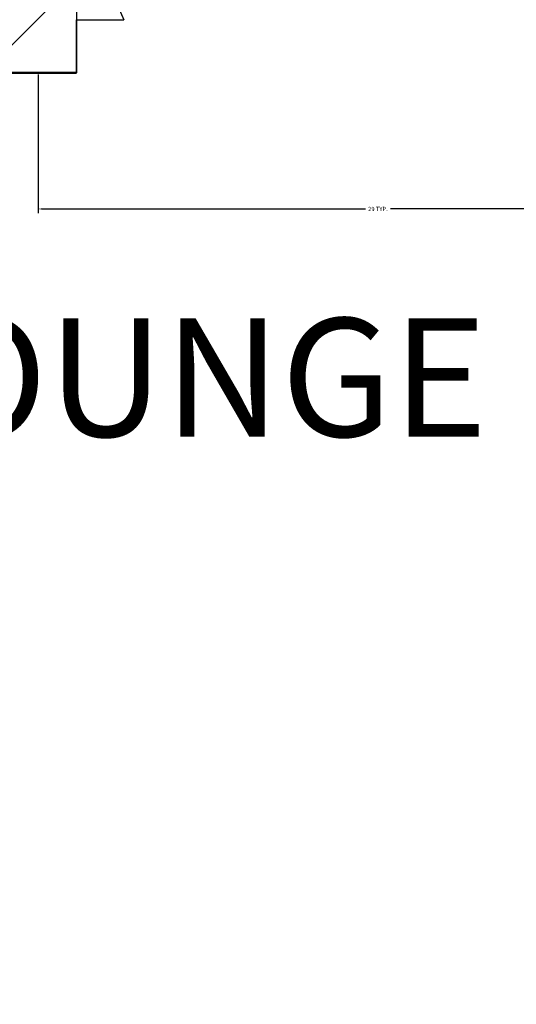
# Model space of a CAD drawing. Units: inches. Extents: x 963 to 2075, y 289 to 2657.
# Tile 64 of 98: x 1224 to 1245, y 2284 to 2325. Entities that reach past the tile are written whole.
import ezdxf

# ---------------------------------------------------------------- set-up
doc = ezdxf.new("R2010")
doc.units = ezdxf.units.IN
for name, color, linetype, lineweight in [('A-ANNO-DIMS', 2, 'Continuous', 18), ('A-AREA-IDEN', 7, 'Continuous', 18), ('A-DOOR', 4, 'Continuous', 25), ('A-WALL', 7, 'Continuous', 50), ('A-WALL-PATT', 8, 'Continuous', 13)]:
    doc.layers.add(name, color=color, linetype=linetype, lineweight=lineweight)
doc.styles.get("Standard").update_dxf_attribs({"font": 'arial.ttf'})
doc.dimstyles.get("Standard").update_dxf_attribs({"dimtxt": 0.18, "dimasz": 0.18, "dimexe": 0.18, "dimexo": 0.0625, "dimgap": 0.09, "dimtad": 0, "dimtih": 1, "dimtoh": 1, "dimdec": 4, "dimzin": 0, "dimdsep": 46, "dimtxsty": 'Standard', "dimcen": 0.09, "dimadec": 0, "dimazin": 0, "dimtfac": 1, "dimtdec": 4, "dimtofl": 0, "dimtmove": 0, "dimatfit": 3, "dimfxl": 1, "dimtolj": 1, "dimtzin": 0, "dimarcsym": 0})

# ---------------------------------------------------------------- blocks, each defined once
blk = doc.blocks.new('DOOR-1')
for p, q in [((25.385, 2.25), (25.385, 38.25)), ((0.325, 4.5), (0.325, 0)), ((27.385, 4.5), (27.385, 0)), ((0.325, 0), (0.325, 2.25)), ((0.325, 2.25), (2.325, 2.25)), ((27.385, 2.25), (25.385, 2.25)), ((27.385, 0), (27.385, 2.25))]:
    blk.add_line(p, q)
blk.add_arc((25.385, 12.864), 25.386, 90, 204.7158)
blk = doc.blocks.new('*D31')
at = {"layer": 'A-ANNO-DIMS', "color": 0, "lineweight": -2, "transparency": 16777216}
for p, q in [((1225.036, 2322.755), (1225.036, 2316.9)), ((1253.714, 2322.755), (1253.714, 2316.9)), ((1225.216, 2317.08), (1238.845, 2317.08)), ((1253.534, 2317.08), (1239.904, 2317.08))]:
    blk.add_line(p, q, dxfattribs=at)
at = {"layer": 'A-ANNO-DIMS', "color": 0, "transparency": 16777216}
for points in [[(1225.216, 2317.11), (1225.216, 2317.05), (1225.036, 2317.08)], [(1253.534, 2317.11), (1253.534, 2317.05), (1253.714, 2317.08)]]:
    blk.add_solid(points, dxfattribs=at)
at = {"layer": 'Defpoints', "color": 0, "transparency": 16777216}
for p in [(1225.036, 2322.818), (1253.714, 2322.818), (1253.714, 2317.08)]:
    blk.add_point(p, dxfattribs=at)
at = {"layer": 'A-ANNO-DIMS', "color": 0, "transparency": 16777216, "insert": (1239.375, 2317.08), "char_height": 0.18, "attachment_point": 5}
blk.add_mtext('\\A1;29 TYP.', dxfattribs=at)

msp = doc.modelspace()

# ---------------------------------------------------------------- hatches: boundary and pattern name
at = {"layer": 'A-WALL-PATT'}
h = msp.add_hatch(dxfattribs=at)
h.set_pattern_fill('ANSI32', color=256)
h.paths.add_polyline_path([(1296.922, 2558.318), (1203.922, 2558.318), (1203.922, 2493.818), (1191.533, 2493.818), (1191.533, 2489.318), (1211.063, 2489.318), (1211.063, 2492.02), (1211.063, 2493.818), (1208.422, 2493.818), (1208.422, 2553.818), (1292.422, 2553.818), (1292.422, 2538.863), (1296.922, 2538.863)])
h.paths.add_polyline_path([(1442.422, 2558.318), (1349.422, 2558.318), (1349.422, 2538.943), (1353.922, 2538.943), (1353.922, 2553.818), (1437.922, 2553.818), (1437.922, 2493.818), (1434.542, 2493.818), (1434.542, 2489.318), (1448.311, 2489.318), (1448.311, 2491.568), (1448.311, 2493.818), (1442.422, 2493.818)])
h.paths.add_polyline_path([(1415.554, 2491.568), (1415.554, 2493.818), (1340.941, 2493.818), (1340.941, 2489.318), (1371.922, 2489.318), (1371.922, 2378.318), (1367.596, 2378.318), (1367.596, 2373.818), (1371.922, 2373.818), (1371.922, 2355.185), (1376.422, 2355.185), (1376.422, 2489.318), (1415.554, 2489.318)])
h.paths.add_polyline_path([(1304.941, 2491.568), (1304.941, 2493.818), (1296.922, 2493.818), (1296.922, 2514.863), (1292.422, 2514.863), (1292.422, 2493.818), (1232.808, 2493.818), (1232.808, 2489.318), (1256.422, 2489.318), (1256.422, 2327.318), (1253.714, 2327.318), (1253.714, 2322.818), (1328.422, 2322.818), (1328.422, 2331.147), (1323.922, 2331.147), (1323.922, 2327.318), (1260.922, 2327.318), (1260.922, 2373.818), (1323.922, 2373.818), (1323.922, 2357.812), (1328.422, 2357.812), (1328.422, 2373.818), (1346.007, 2373.818), (1346.007, 2376.068), (1346.007, 2378.318), (1260.922, 2378.318), (1260.922, 2489.318), (1304.941, 2489.318)])
h.paths.add_polyline_path([(1226.654, 2327.318), (1124.422, 2327.318), (1124.422, 2347.447), (1119.922, 2347.447), (1119.922, 2322.818), (1163.422, 2322.818), (1163.422, 2305.435), (1165.672, 2305.435), (1167.922, 2305.435), (1167.922, 2322.818), (1226.654, 2322.818), (1226.654, 2325.068)])
h.paths.add_polyline_path([(1095.922, 2489.318), (1124.422, 2489.318), (1131.533, 2489.318), (1131.533, 2491.568), (1131.533, 2493.818), (1119.922, 2493.818), (1091.422, 2493.818), (1091.422, 2417.318), (1095.922, 2417.318), (1119.922, 2417.318), (1119.922, 2407.447), (1124.422, 2407.447), (1124.422, 2421.818), (1095.922, 2421.818)])
h.paths.add_polyline_path([(1512.922, 2558.318), (1508.422, 2558.318), (1508.422, 2493.818), (1503.401, 2493.818), (1503.401, 2489.318), (1508.422, 2489.318), (1508.422, 2327.318), (1376.422, 2327.318), (1376.422, 2330.273), (1371.922, 2330.273), (1371.922, 2298.744), (1376.422, 2298.744), (1376.422, 2322.818), (1508.422, 2322.818), (1508.422, 2165.318), (1504.255, 2165.318), (1504.255, 2160.818), (1508.422, 2160.818), (1508.422, 2108.318), (1512.922, 2108.318), (1512.922, 2160.818), (1516.182, 2160.818), (1516.182, 2163.068), (1516.182, 2165.318), (1512.922, 2165.318), (1512.922, 2322.818), (1644.922, 2322.818), (1644.922, 2298.744), (1649.422, 2298.744), (1649.422, 2322.818), (1649.422, 2330.944), (1647.172, 2330.944), (1644.922, 2330.944), (1644.922, 2327.318), (1512.922, 2327.318), (1512.922, 2489.318), (1516.759, 2489.318), (1516.759, 2491.568), (1516.759, 2493.818), (1512.922, 2493.818)])
h.paths.add_polyline_path([(1671.922, 2558.318), (1578.922, 2558.318), (1578.922, 2493.818), (1573.526, 2493.818), (1573.526, 2489.318), (1586.537, 2489.318), (1586.537, 2491.568), (1586.537, 2493.818), (1583.422, 2493.818), (1583.422, 2553.818), (1667.422, 2553.818), (1667.422, 2541.109), (1671.922, 2541.109)])
h.paths.add_polyline_path([(1681.257, 2493.818), (1671.922, 2493.818), (1671.922, 2517.109), (1667.422, 2517.109), (1667.422, 2493.818), (1610.218, 2493.818), (1610.218, 2489.318), (1644.922, 2489.318), (1644.922, 2357.865), (1649.422, 2357.865), (1649.422, 2373.818), (1652.203, 2373.818), (1652.203, 2375.827), (1652.203, 2378.318), (1649.422, 2378.318), (1649.422, 2489.318), (1681.257, 2489.318), (1681.257, 2491.568)])
h.paths.add_polyline_path([(1821.922, 2558.318), (1728.922, 2558.318), (1728.922, 2541), (1733.422, 2541), (1733.422, 2553.818), (1817.422, 2553.818), (1817.422, 2493.818), (1813.507, 2493.818), (1813.507, 2489.318), (1830.078, 2489.318), (1830.078, 2491.568), (1830.078, 2493.818), (1821.922, 2493.818)])
h.paths.add_polyline_path([(1794.244, 2493.818), (1717.257, 2493.818), (1717.257, 2489.318), (1760.422, 2489.318), (1760.422, 2378.318), (1674.401, 2378.318), (1674.401, 2373.818), (1692.922, 2373.818), (1692.922, 2356.954), (1697.422, 2356.954), (1697.422, 2373.818), (1760.422, 2373.818), (1760.422, 2327.318), (1697.422, 2327.318), (1697.422, 2333.341), (1692.922, 2333.341), (1692.922, 2322.818), (1768.037, 2322.818), (1768.037, 2325.068), (1768.037, 2327.318), (1764.922, 2327.318), (1764.922, 2489.318), (1794.244, 2489.318)])
h.paths.add_polyline_path([(1733.422, 2517), (1728.922, 2517), (1728.922, 2493.818), (1733.422, 2493.818)], flags=17)
h.paths.add_polyline_path([(1929.922, 2493.818), (1890.078, 2493.818), (1890.078, 2489.318), (1896.922, 2489.318), (1925.422, 2489.318), (1925.422, 2421.818), (1896.922, 2421.818), (1896.922, 2408.318), (1901.422, 2408.318), (1901.422, 2417.318), (1925.422, 2417.318), (1929.922, 2417.318)])
h.paths.add_polyline_path([(1901.422, 2348.318), (1896.922, 2348.318), (1896.922, 2327.318), (1800.423, 2327.318), (1800.423, 2322.818), (1853.422, 2322.818), (1853.422, 2309.453), (1857.922, 2309.453), (1857.922, 2322.818), (1901.422, 2322.818)])
h.paths.add_polyline_path([(1857.922, 2249.453), (1853.422, 2249.453), (1853.422, 2214.818), (1686.309, 2214.818), (1686.309, 2210.318), (1853.422, 2210.318), (1853.422, 2202.134), (1857.922, 2202.134), (1857.922, 2210.318)])
h.paths.add_polyline_path([(1857.922, 2142.134), (1853.422, 2142.134), (1853.422, 2115.422), (1841.422, 2115.422), (1841.422, 2088.531), (1841.422, 2046.949), (1845.922, 2046.949), (1845.922, 2110.922), (1905.922, 2110.922), (1905.922, 2092.517), (1910.422, 2092.517), (1910.422, 2115.422), (1857.922, 2115.422)])
h.paths.add_polyline_path([(1532.436, 1482.342), (1573.456, 1482.342), (1573.456, 1501), (1532.436, 1501)], flags=9)
h.paths.add_polyline_path([(1438.658, 1486.302), (1479.678, 1486.302), (1479.678, 1504.96), (1438.658, 1504.96)], flags=9)
h.paths.add_polyline_path([(1411.215, 1365.308), (1659.139, 1365.308), (1659.139, 1402.401), (1411.215, 1402.401)], flags=9)
h.paths.add_polyline_path([(1185.671, 2296.298), (1248.16, 2296.298), (1248.16, 2314.955), (1185.671, 2314.955)], flags=9)
h.paths.add_polyline_path([(1177.31, 2187.35), (1216.15, 2187.35), (1216.15, 2206.007), (1177.31, 2206.007)], flags=9)
h.paths.add_polyline_path([(1295.101, 1602.083), (1328.26, 1602.083), (1328.26, 1620.741), (1295.101, 1620.741)], flags=9)
h.paths.add_polyline_path([(1525.126, 2005.99), (1558.39, 2005.99), (1558.39, 2024.648), (1525.126, 2024.648)], flags=9)
h.paths.add_polyline_path([(1459.606, 1977.125), (1472.195, 1977.125), (1472.195, 1987.429), (1459.606, 1987.429)], flags=9)
h.paths.add_polyline_path([(1467.815, 2053.676), (1480.018, 2053.676), (1480.018, 2063.979), (1467.815, 2063.979)], flags=9)
h.paths.add_polyline_path([(1555.184, 2119.02), (1584.563, 2119.02), (1584.563, 2137.678), (1555.184, 2137.678)], flags=25)
h.paths.add_polyline_path([(1405.389, 2115.291), (1444.478, 2115.291), (1444.478, 2133.948), (1405.389, 2133.948)], flags=25)
h.paths.add_polyline_path([(1698.482, 2004.259), (1727.695, 2004.259), (1727.695, 2022.916), (1698.482, 2022.916)], flags=9)
h.paths.add_polyline_path([(1612.158, 1972.855), (1629.016, 1972.855), (1629.016, 1983.159), (1612.158, 1983.159)], flags=9)
h.paths.add_polyline_path([(1608.289, 2060.036), (1625.147, 2060.036), (1625.147, 2070.34), (1608.289, 2070.34)], flags=9)
h.paths.add_polyline_path([(1527.954, 1684.402), (1566.795, 1684.402), (1566.795, 1703.06), (1527.954, 1703.06)], flags=9)
h.paths.add_polyline_path([(1422.792, 1683.59), (1461.633, 1683.59), (1461.633, 1702.247), (1422.792, 1702.247)], flags=9)
h.paths.add_polyline_path([(1531.262, 1732.459), (1574.015, 1732.459), (1574.015, 1751.116), (1531.262, 1751.116)], flags=9)
h.paths.add_polyline_path([(1402.872, 1732.845), (1439.799, 1732.845), (1439.799, 1751.502), (1402.872, 1751.502)], flags=9)
h.paths.add_polyline_path([(1243.122, 1923.132), (1281.962, 1923.132), (1281.962, 1941.79), (1243.122, 1941.79)], flags=9)
h.paths.add_polyline_path([(1181.752, 1792.268), (1244.241, 1792.268), (1244.241, 1810.926), (1181.752, 1810.926)], flags=9)
h.paths.add_polyline_path([(1265.822, 1670.3), (1316.071, 1670.3), (1316.071, 1688.957), (1265.822, 1688.957)], flags=9)
h.paths.add_polyline_path([(1140.263, 1676.054), (1179.104, 1676.054), (1179.104, 1694.711), (1140.263, 1694.711)], flags=9)
h.paths.add_polyline_path([(1107.49, 1490.889), (1143.374, 1490.889), (1143.374, 1509.546), (1107.49, 1509.546)], flags=9)
h.paths.add_polyline_path([(1217.584, 1483.899), (1246.741, 1483.899), (1246.741, 1502.556), (1217.584, 1502.556)], flags=9)
h.paths.add_polyline_path([(1389.21, 1486.919), (1418.367, 1486.919), (1418.367, 1505.576), (1389.21, 1505.576)], flags=9)
h.paths.add_polyline_path([(1672.208, 1602.083), (1705.366, 1602.083), (1705.366, 1620.741), (1672.208, 1620.741)], flags=9)
h.paths.add_polyline_path([(1752.082, 1522.638), (1781.24, 1522.638), (1781.24, 1541.295), (1752.082, 1541.295)], flags=9)
h.paths.add_polyline_path([(1848.275, 1491.26), (1884.158, 1491.26), (1884.158, 1509.918), (1848.275, 1509.918)], flags=9)
h.paths.add_polyline_path([(1822.47, 1685.62), (1861.31, 1685.62), (1861.31, 1704.278), (1822.47, 1704.278)], flags=9)
h.paths.add_polyline_path([(1713.195, 1672.232), (1763.444, 1672.232), (1763.444, 1690.889), (1713.195, 1690.889)], flags=9)
h.paths.add_polyline_path([(1736.619, 1790.578), (1799.109, 1790.578), (1799.109, 1809.235), (1736.619, 1809.235)], flags=9)
h.paths.add_polyline_path([(1691.491, 1916.355), (1730.332, 1916.355), (1730.332, 1935.013), (1691.491, 1935.013)], flags=9)
h.paths.add_polyline_path([(1764.872, 1973.922), (1794.306, 1973.922), (1794.306, 1992.58), (1764.872, 1992.58)], flags=9)
h.paths.add_polyline_path([(1767.854, 2034.017), (1797.288, 2034.017), (1797.288, 2052.674), (1767.854, 2052.674)], flags=9)
h.paths.add_polyline_path([(1851.593, 2060.331), (1880.751, 2060.331), (1880.751, 2078.989), (1851.593, 2078.989)], flags=25)
h.paths.add_polyline_path([(1688.491, 2086.874), (1727.332, 2086.874), (1727.332, 2105.531), (1688.491, 2105.531)], flags=9)
h.paths.add_polyline_path([(1537.743, 2293.581), (1580.495, 2293.581), (1580.495, 2312.239), (1537.743, 2312.239)], flags=25)
h.paths.add_polyline_path([(1425.587, 2296.109), (1468.34, 2296.109), (1468.34, 2314.766), (1425.587, 2314.766)], flags=25)
h.paths.add_polyline_path([(1278.518, 2004.184), (1307.72, 2004.184), (1307.72, 2022.841), (1278.518, 2022.841)], flags=9)
h.paths.add_polyline_path([(1193.282, 1973.635), (1222.715, 1973.635), (1222.715, 1992.292), (1193.282, 1992.292)], flags=9)
h.paths.add_polyline_path([(1192.411, 2040.577), (1221.845, 2040.577), (1221.845, 2059.234), (1192.411, 2059.234)], flags=9)
h.paths.add_polyline_path([(1130.603, 1951.393), (1159.76, 1951.393), (1159.76, 1970.05), (1130.603, 1970.05)], flags=9)
h.paths.add_polyline_path([(1132.827, 2052.494), (1161.984, 2052.494), (1161.984, 2071.151), (1132.827, 2071.151)], flags=9)
h.paths.add_polyline_path([(1265.128, 2334.619), (1315.377, 2334.619), (1315.377, 2353.277), (1265.128, 2353.277)], flags=25)
h.paths.add_polyline_path([(1136.741, 2330.785), (1175.582, 2330.785), (1175.582, 2349.443), (1136.741, 2349.443)], flags=9)
h.paths.add_polyline_path([(1287.422, 2417.204), (1320.58, 2417.204), (1320.58, 2435.861), (1287.422, 2435.861)], flags=25)
h.paths.add_polyline_path([(1430.988, 2329.159), (1469.828, 2329.159), (1469.828, 2347.816), (1430.988, 2347.816)], flags=25)
h.paths.add_polyline_path([(1525.424, 2329.213), (1564.264, 2329.213), (1564.264, 2347.87), (1525.424, 2347.87)], flags=25)
h.paths.add_polyline_path([(1684.525, 2382.799), (1717.683, 2382.799), (1717.683, 2401.457), (1684.525, 2401.457)], flags=25)
h.paths.add_polyline_path([(1704.805, 2340.293), (1755.054, 2340.293), (1755.054, 2358.95), (1704.805, 2358.95)], flags=25)
h.paths.add_polyline_path([(1694.113, 2287.757), (1756.602, 2287.757), (1756.602, 2306.414), (1694.113, 2306.414)], flags=9)
h.paths.add_polyline_path([(1815.778, 2329.861), (1854.618, 2329.861), (1854.618, 2348.518), (1815.778, 2348.518)], flags=9)
h.paths.add_polyline_path([(1842.873, 2514.256), (1878.756, 2514.256), (1878.756, 2532.914), (1842.873, 2532.914)], flags=9)
h.paths.add_polyline_path([(1769.513, 2531.447), (1798.671, 2531.447), (1798.671, 2550.104), (1769.513, 2550.104)], flags=25)
h.paths.add_polyline_path([(1594.772, 2518.468), (1623.93, 2518.468), (1623.93, 2537.125), (1594.772, 2537.125)], flags=25)
h.paths.add_polyline_path([(1520.723, 2516.185), (1556.606, 2516.185), (1556.606, 2534.842), (1520.723, 2534.842)], flags=25)
h.paths.add_polyline_path([(1464.456, 2516.694), (1500.34, 2516.694), (1500.34, 2535.351), (1464.456, 2535.351)], flags=25)
h.paths.add_polyline_path([(1365.696, 2528.97), (1394.854, 2528.97), (1394.854, 2547.627), (1365.696, 2547.627)], flags=25)
h.paths.add_polyline_path([(1222.838, 2516.231), (1251.995, 2516.231), (1251.995, 2534.889), (1222.838, 2534.889)], flags=25)
h.paths.add_polyline_path([(1104.545, 2509.6), (1140.429, 2509.6), (1140.429, 2528.257), (1104.545, 2528.257)], flags=9)
h = msp.add_hatch(dxfattribs=at)
h.set_pattern_fill('ANSI32', color=256)
h.paths.add_polyline_path([(1335.968, 2212.568), (1335.968, 2214.818), (1167.922, 2214.818), (1167.922, 2245.435), (1163.422, 2245.435), (1163.422, 2210.318), (1163.422, 2194.812), (1167.922, 2194.812), (1167.922, 2210.318), (1335.968, 2210.318)])
h.paths.add_polyline_path([(1532.436, 1482.342), (1573.456, 1482.342), (1573.456, 1501), (1532.436, 1501)], flags=9)
h.paths.add_polyline_path([(1438.658, 1486.302), (1479.678, 1486.302), (1479.678, 1504.96), (1438.658, 1504.96)], flags=9)
h.paths.add_polyline_path([(1411.215, 1365.308), (1659.139, 1365.308), (1659.139, 1402.401), (1411.215, 1402.401)], flags=9)
h.paths.add_polyline_path([(1185.671, 2296.298), (1248.16, 2296.298), (1248.16, 2314.955), (1185.671, 2314.955)], flags=9)
h.paths.add_polyline_path([(1177.31, 2187.35), (1216.15, 2187.35), (1216.15, 2206.007), (1177.31, 2206.007)], flags=9)
h.paths.add_polyline_path([(1295.101, 1602.083), (1328.26, 1602.083), (1328.26, 1620.741), (1295.101, 1620.741)], flags=9)
h.paths.add_polyline_path([(1525.126, 2005.99), (1558.39, 2005.99), (1558.39, 2024.648), (1525.126, 2024.648)], flags=9)
h.paths.add_polyline_path([(1459.606, 1977.125), (1472.195, 1977.125), (1472.195, 1987.429), (1459.606, 1987.429)], flags=9)
h.paths.add_polyline_path([(1467.815, 2053.676), (1480.018, 2053.676), (1480.018, 2063.979), (1467.815, 2063.979)], flags=9)
h.paths.add_polyline_path([(1555.184, 2119.02), (1584.563, 2119.02), (1584.563, 2137.678), (1555.184, 2137.678)], flags=9)
h.paths.add_polyline_path([(1405.389, 2115.291), (1444.478, 2115.291), (1444.478, 2133.948), (1405.389, 2133.948)], flags=9)
h.paths.add_polyline_path([(1698.482, 2004.259), (1727.695, 2004.259), (1727.695, 2022.916), (1698.482, 2022.916)], flags=9)
h.paths.add_polyline_path([(1612.158, 1972.855), (1629.016, 1972.855), (1629.016, 1983.159), (1612.158, 1983.159)], flags=9)
h.paths.add_polyline_path([(1608.289, 2060.036), (1625.147, 2060.036), (1625.147, 2070.34), (1608.289, 2070.34)], flags=9)
h.paths.add_polyline_path([(1527.954, 1684.402), (1566.795, 1684.402), (1566.795, 1703.06), (1527.954, 1703.06)], flags=9)
h.paths.add_polyline_path([(1422.792, 1683.59), (1461.633, 1683.59), (1461.633, 1702.247), (1422.792, 1702.247)], flags=9)
h.paths.add_polyline_path([(1531.262, 1732.459), (1574.015, 1732.459), (1574.015, 1751.116), (1531.262, 1751.116)], flags=9)
h.paths.add_polyline_path([(1402.872, 1732.845), (1439.799, 1732.845), (1439.799, 1751.502), (1402.872, 1751.502)], flags=9)
h.paths.add_polyline_path([(1243.122, 1923.132), (1281.962, 1923.132), (1281.962, 1941.79), (1243.122, 1941.79)], flags=9)
h.paths.add_polyline_path([(1181.752, 1792.268), (1244.241, 1792.268), (1244.241, 1810.926), (1181.752, 1810.926)], flags=9)
h.paths.add_polyline_path([(1265.822, 1670.3), (1316.071, 1670.3), (1316.071, 1688.957), (1265.822, 1688.957)], flags=9)
h.paths.add_polyline_path([(1140.263, 1676.054), (1179.104, 1676.054), (1179.104, 1694.711), (1140.263, 1694.711)], flags=9)
h.paths.add_polyline_path([(1107.49, 1490.889), (1143.374, 1490.889), (1143.374, 1509.546), (1107.49, 1509.546)], flags=9)
h.paths.add_polyline_path([(1217.584, 1483.899), (1246.741, 1483.899), (1246.741, 1502.556), (1217.584, 1502.556)], flags=9)
h.paths.add_polyline_path([(1389.21, 1486.919), (1418.367, 1486.919), (1418.367, 1505.576), (1389.21, 1505.576)], flags=9)
h.paths.add_polyline_path([(1672.208, 1602.083), (1705.366, 1602.083), (1705.366, 1620.741), (1672.208, 1620.741)], flags=9)
h.paths.add_polyline_path([(1752.082, 1522.638), (1781.24, 1522.638), (1781.24, 1541.295), (1752.082, 1541.295)], flags=9)
h.paths.add_polyline_path([(1848.275, 1491.26), (1884.158, 1491.26), (1884.158, 1509.918), (1848.275, 1509.918)], flags=9)
h.paths.add_polyline_path([(1822.47, 1685.62), (1861.31, 1685.62), (1861.31, 1704.278), (1822.47, 1704.278)], flags=9)
h.paths.add_polyline_path([(1713.195, 1672.232), (1763.444, 1672.232), (1763.444, 1690.889), (1713.195, 1690.889)], flags=9)
h.paths.add_polyline_path([(1736.619, 1790.578), (1799.109, 1790.578), (1799.109, 1809.235), (1736.619, 1809.235)], flags=9)
h.paths.add_polyline_path([(1691.491, 1916.355), (1730.332, 1916.355), (1730.332, 1935.013), (1691.491, 1935.013)], flags=9)
h.paths.add_polyline_path([(1764.872, 1973.922), (1794.306, 1973.922), (1794.306, 1992.58), (1764.872, 1992.58)], flags=9)
h.paths.add_polyline_path([(1767.854, 2034.017), (1797.288, 2034.017), (1797.288, 2052.674), (1767.854, 2052.674)], flags=9)
h.paths.add_polyline_path([(1851.593, 2060.331), (1880.751, 2060.331), (1880.751, 2078.989), (1851.593, 2078.989)], flags=9)
h.paths.add_polyline_path([(1688.491, 2086.874), (1727.332, 2086.874), (1727.332, 2105.531), (1688.491, 2105.531)], flags=9)
h.paths.add_polyline_path([(1537.743, 2293.581), (1580.495, 2293.581), (1580.495, 2312.239), (1537.743, 2312.239)], flags=9)
h.paths.add_polyline_path([(1425.587, 2296.109), (1468.34, 2296.109), (1468.34, 2314.766), (1425.587, 2314.766)], flags=9)
h.paths.add_polyline_path([(1278.518, 2004.184), (1307.72, 2004.184), (1307.72, 2022.841), (1278.518, 2022.841)], flags=9)
h.paths.add_polyline_path([(1193.282, 1973.635), (1222.715, 1973.635), (1222.715, 1992.292), (1193.282, 1992.292)], flags=9)
h.paths.add_polyline_path([(1192.411, 2040.577), (1221.845, 2040.577), (1221.845, 2059.234), (1192.411, 2059.234)], flags=9)
h.paths.add_polyline_path([(1130.603, 1951.393), (1159.76, 1951.393), (1159.76, 1970.05), (1130.603, 1970.05)], flags=9)
h.paths.add_polyline_path([(1132.827, 2052.494), (1161.984, 2052.494), (1161.984, 2071.151), (1132.827, 2071.151)], flags=9)
h.paths.add_polyline_path([(1265.128, 2334.619), (1315.377, 2334.619), (1315.377, 2353.277), (1265.128, 2353.277)], flags=9)
h.paths.add_polyline_path([(1136.741, 2330.785), (1175.582, 2330.785), (1175.582, 2349.443), (1136.741, 2349.443)], flags=9)
h.paths.add_polyline_path([(1287.422, 2417.204), (1320.58, 2417.204), (1320.58, 2435.861), (1287.422, 2435.861)], flags=9)
h.paths.add_polyline_path([(1430.988, 2329.159), (1469.828, 2329.159), (1469.828, 2347.816), (1430.988, 2347.816)], flags=9)
h.paths.add_polyline_path([(1525.424, 2329.213), (1564.264, 2329.213), (1564.264, 2347.87), (1525.424, 2347.87)], flags=9)
h.paths.add_polyline_path([(1684.525, 2382.799), (1717.683, 2382.799), (1717.683, 2401.457), (1684.525, 2401.457)], flags=9)
h.paths.add_polyline_path([(1704.805, 2340.293), (1755.054, 2340.293), (1755.054, 2358.95), (1704.805, 2358.95)], flags=9)
h.paths.add_polyline_path([(1694.113, 2287.757), (1756.602, 2287.757), (1756.602, 2306.414), (1694.113, 2306.414)], flags=9)
h.paths.add_polyline_path([(1815.778, 2329.861), (1854.618, 2329.861), (1854.618, 2348.518), (1815.778, 2348.518)], flags=9)
h.paths.add_polyline_path([(1842.873, 2514.256), (1878.756, 2514.256), (1878.756, 2532.914), (1842.873, 2532.914)], flags=9)
h.paths.add_polyline_path([(1769.513, 2531.447), (1798.671, 2531.447), (1798.671, 2550.104), (1769.513, 2550.104)], flags=9)
h.paths.add_polyline_path([(1594.772, 2518.468), (1623.93, 2518.468), (1623.93, 2537.125), (1594.772, 2537.125)], flags=9)
h.paths.add_polyline_path([(1520.723, 2516.185), (1556.606, 2516.185), (1556.606, 2534.842), (1520.723, 2534.842)], flags=9)
h.paths.add_polyline_path([(1464.456, 2516.694), (1500.34, 2516.694), (1500.34, 2535.351), (1464.456, 2535.351)], flags=9)
h.paths.add_polyline_path([(1365.696, 2528.97), (1394.854, 2528.97), (1394.854, 2547.627), (1365.696, 2547.627)], flags=9)
h.paths.add_polyline_path([(1222.838, 2516.231), (1251.995, 2516.231), (1251.995, 2534.889), (1222.838, 2534.889)], flags=9)
h.paths.add_polyline_path([(1104.545, 2509.6), (1140.429, 2509.6), (1140.429, 2528.257), (1104.545, 2528.257)], flags=9)

# ---------------------------------------------------------------- linework, layer by layer
at = {"layer": 'A-WALL'}
msp.add_line((1167.922, 2322.818), (1226.654, 2322.818), dxfattribs=at)

# ---------------------------------------------------------------- block references
at = {"layer": 'A-DOOR'}
msp.add_blockref('DOOR-1', (1226.329, 2322.818), dxfattribs=at)

# ---------------------------------------------------------------- texts
at = {"layer": 'A-AREA-IDEN', "insert": (1187.681, 2312.47), "char_height": 5, "attachment_point": 1}
msp.add_mtext_dynamic_manual_height_columns('DINING / LOUNGE\\P17\'0"x9\'0"', width=166.99497, gutter_width=12.5, heights=[0], dxfattribs=at)

# ---------------------------------------------------------------- dimensions: what is measured, and where the dimension line sits
at = {"layer": 'A-ANNO-DIMS'}
dim = msp.add_linear_dim(base=(1253.714, 2317.08), p1=(1225.036, 2322.818), p2=(1253.714, 2322.818), text='<> TYP.', dimstyle='Standard', override={"dimdec": 0, "dimlfac": 1, "dimrnd": 0, "dimzin": 0, "dimdsep": 46, "dimlunit": 2}, dxfattribs=at)
dim.commit()
dim.dimension.update_dxf_attribs({"geometry": '*D31', "text_midpoint": (1239.375, 2317.08)})

doc.saveas('drawing.dxf')
